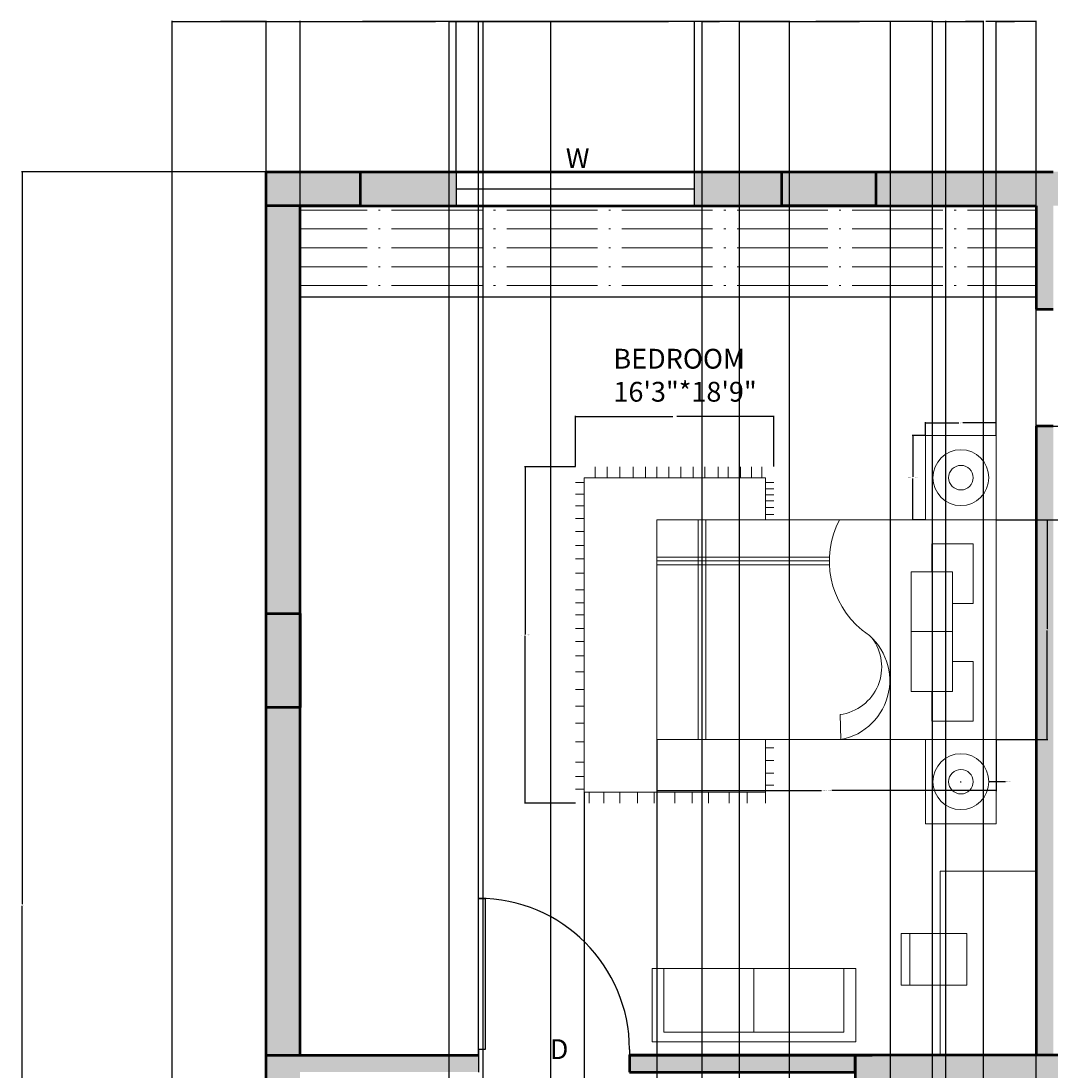
# Model space of a CAD drawing. Units: inches. Extents: x 2494 to 2908, y 1051 to 1885.
# Tile 6 of 7: x 2494 to 2767, y 1607 to 1885. Entities that reach past the tile are written whole.
import ezdxf

# ---------------------------------------------------------------- set-up
doc = ezdxf.new("R2010")
doc.units = ezdxf.units.IN
for name, color, linetype, lineweight in [('A-ANNO-DIMS', 2, 'Continuous', 18), ('A-ANNO-IDEN', 130, 'Continuous', 18), ('A-AREA-IDEN', 130, 'Continuous', 18), ('A-COLS-PATT', 200, 'Continuous', 13), ('A-FLOR-CASE', 230, 'Continuous', 25), ('A-FURN-PATT', 230, 'Continuous', 13), ('A-WALL-PATT', 140, 'Continuous', 13), ('COLUMN', 200, 'Continuous', 50), ('DOOR', 50, 'Continuous', 25), ('FUR', 230, 'Continuous', 18), ('WALL', 140, 'Continuous', 50), ('WIND', 210, 'Continuous', 25)]:
    doc.layers.add(name, color=color, linetype=linetype, lineweight=lineweight)
doc.styles.get("Standard").update_dxf_attribs({"font": 'arial.ttf'})
doc.dimstyles.get("Standard").update_dxf_attribs({"dimtxt": 0.18, "dimasz": 0.18, "dimexe": 0.18, "dimexo": 0.0625, "dimgap": 0.09, "dimtad": 0, "dimtih": 1, "dimtoh": 1, "dimdec": 4, "dimzin": 0, "dimdsep": 46, "dimtxsty": 'Standard', "dimcen": 0.09, "dimadec": 0, "dimazin": 0, "dimtfac": 1, "dimtdec": 4, "dimtofl": 0, "dimtmove": 0, "dimatfit": 3, "dimfxl": 1, "dimtolj": 1, "dimtzin": 0, "dimarcsym": 0})

# ---------------------------------------------------------------- blocks, each defined once
blk = doc.blocks.new('*U2')
for p, q in [((0, 0), (0, -6)), ((40, 0), (40, -6))]:
    blk.add_line(p, q)
blk.add_lwpolyline([(0, 0), (0, 40), (1.75, 40), (1.75, 0)], close=True)
blk.add_arc((0, 0), 40, 0, 90)
blk = doc.blocks.new('BED-DOUBLE')
for p, q in [((10.93, 58.24), (10.93, 0)), ((11.93, 58.24), (11.93, 0)), ((12.93, 58.24), (12.93, 0)), ((45.66, 48.34), (0, 48.34)), ((45.66, 47.34), (0, 47.34)), ((45.66, 46.34), (0, 46.34)), ((67.33, 28.6), (78.31, 28.6)), ((48.68, 0), (48.5, 6.63))]:
    blk.add_line(p, q)
for points in [[(89.88, 0), (0, 0), (0, 58.24), (89.88, 58.24)], [(78.31, 44.44), (67.33, 44.44), (67.33, 12.76), (78.31, 12.76)], [(67.33, 28.6), (78.31, 28.6), (78.31, 44.44), (67.33, 44.44)], [(67.33, 12.76), (78.31, 12.76), (78.31, 28.6), (67.33, 28.6)]]:
    blk.add_lwpolyline(points, close=True)
for points in [[(78.31, 36.06), (83.8, 36.06), (83.8, 51.9), (72.82, 51.9), (72.82, 44.44)], [(72.82, 12.76), (72.82, 4.84), (83.8, 4.84), (83.8, 20.68), (78.31, 20.68)]]:
    blk.add_lwpolyline(points)
for centre, radius, start, end in [((69.31, 47.34), 23.65, 152.5545, 230.8062), ((45.78, 15.63), 15.89, 280.497, 57.3115), ((46.81, 19.24), 12.73, 277.6511, 37.2925)]:
    blk.add_arc(centre, radius, start, end)
blk = doc.blocks.new('NIGHTSTAND-WITH-LAMP')
blk.add_lwpolyline([(18.73, 0), (0, 0), (0, 22.3), (18.73, 22.3)], close=True)
for radius in [7.4, 3.25]:
    blk.add_circle((9.36, 11.15), radius)
blk = doc.blocks.new('RUG-BEDROOM-FRINGED')
for p, q in [((5.18, 86.18), (5.18, 89.12)), ((8.36, 86.18), (8.36, 89.12)), ((11.73, 86.18), (11.73, 89.12)), ((15.23, 86.18), (15.23, 89.12)), ((18.48, 86.18), (18.48, 89.12)), ((21.53, 86.18), (21.53, 89.12)), ((24.71, 86.18), (24.71, 89.12)), ((27.86, 86.18), (27.86, 89.12)), ((31.13, 86.18), (31.13, 89.12)), ((34.27, 86.18), (34.27, 89.12)), ((37.78, 86.18), (37.78, 89.12)), ((40.38, 86.18), (40.38, 89.12)), ((43.7, 86.18), (43.7, 89.12)), ((46.57, 86.18), (46.57, 89.12)), ((49.32, 86.18), (49.32, 89.12)), ((0, 84.95), (2.23, 84.95)), ((50.28, 86.18), (2.23, 86.18)), ((2.23, 86.18), (2.23, 2.94)), ((50.28, 75.11), (50.28, 86.18)), ((50.28, 84.95), (52.51, 84.95)), ((0, 81.88), (2.23, 81.88)), ((50.28, 83.33), (52.51, 83.33)), ((50.28, 81.74), (52.51, 81.74)), ((0, 78.8), (2.23, 78.8)), ((50.28, 80.14), (52.51, 80.14)), ((50.28, 78.33), (52.51, 78.33)), ((0, 75.44), (2.23, 75.44)), ((50.28, 76.54), (52.51, 76.54)), ((0, 71.98), (2.23, 71.98)), ((0, 68.3), (2.23, 68.3)), ((0, 64.75), (2.23, 64.75)), ((0, 60.92), (2.23, 60.92)), ((0, 56.55), (2.23, 56.55)), ((0, 53.1), (2.23, 53.1)), ((0, 49.9), (2.23, 49.9)), ((0, 46.27), (2.23, 46.27)), ((0, 42.87), (2.23, 42.87)), ((0, 39.09), (2.23, 39.09)), ((0, 34.84), (2.23, 34.84)), ((0, 30.1), (2.23, 30.1)), ((0, 25.69), (2.23, 25.69)), ((0, 21.25), (2.23, 21.25)), ((50.28, 2.94), (50.28, 16.87)), ((0, 16.29), (2.23, 16.29)), ((50.28, 14.72), (52.51, 14.72)), ((50.28, 11.34), (52.51, 11.34)), ((0, 10.85), (2.23, 10.85)), ((0, 7.08), (2.23, 7.08)), ((50.28, 7.95), (52.51, 7.95)), ((0, 3.73), (2.23, 3.73)), ((2.23, 2.94), (50.28, 2.94)), ((3.63, 0), (3.63, 2.94)), ((7.47, 0), (7.47, 2.94)), ((11.7, 0), (11.7, 2.94)), ((16.39, 0), (16.39, 2.94)), ((20.78, 0), (20.78, 2.94)), ((26.26, 0), (26.26, 2.94)), ((30.86, 0), (30.86, 2.94)), ((35.17, 0), (35.17, 2.94)), ((40.63, 0), (40.63, 2.94)), ((45.48, 0), (45.48, 2.94)), ((50.28, 4.8), (52.51, 4.8)), ((50.28, 0), (50.28, 2.94))]:
    blk.add_line(p, q)
blk = doc.blocks.new('*D12')
at = {"layer": 'A-ANNO-DIMS', "color": 0, "lineweight": -2, "transparency": 16777216}
for p, q in [((2733.86, 1775.26), (2730.39, 1775.26)), ((2730.57, 1775.08), (2730.57, 1764.29)), ((2730.57, 1753.14), (2730.57, 1763.92)), ((2733.86, 1752.96), (2730.39, 1752.96))]:
    blk.add_line(p, q, dxfattribs=at)
at = {"layer": 'A-ANNO-DIMS', "color": 0, "lineweight": 100, "transparency": 16777216}
for points in [[(2730.54, 1775.08), (2730.6, 1775.08), (2730.57, 1775.26)], [(2730.54, 1753.14), (2730.6, 1753.14), (2730.57, 1752.96)]]:
    blk.add_solid(points, dxfattribs=at)
at = {"layer": 'Defpoints', "color": 0, "lineweight": 100, "transparency": 16777216}
for p in [(2730.57, 1775.26), (2733.92, 1775.26), (2733.92, 1752.96)]:
    blk.add_point(p, dxfattribs=at)
at = {"layer": 'A-ANNO-DIMS', "color": 0, "transparency": 16777216, "insert": (2730.57, 1764.11), "char_height": 0.18, "attachment_point": 5}
blk.add_mtext('\\A1;NIGHTSTAND 22 TYP.', dxfattribs=at)
blk = doc.blocks.new('*D13')
at = {"layer": 'A-ANNO-DIMS', "color": 0, "lineweight": -2, "transparency": 16777216}
for p, q in [((2733.92, 1775.32), (2733.92, 1778.78)), ((2734.1, 1778.6), (2742.76, 1778.6)), ((2752.46, 1778.6), (2743.8, 1778.6)), ((2752.64, 1775.32), (2752.64, 1778.78))]:
    blk.add_line(p, q, dxfattribs=at)
at = {"layer": 'A-ANNO-DIMS', "color": 0, "lineweight": 100, "transparency": 16777216}
for points in [[(2734.1, 1778.63), (2734.1, 1778.57), (2733.92, 1778.6)], [(2752.46, 1778.63), (2752.46, 1778.57), (2752.64, 1778.6)]]:
    blk.add_solid(points, dxfattribs=at)
at = {"layer": 'Defpoints', "color": 0, "lineweight": 100, "transparency": 16777216}
for p in [(2752.64, 1778.6), (2733.92, 1775.26), (2752.64, 1775.26)]:
    blk.add_point(p, dxfattribs=at)
at = {"layer": 'A-ANNO-DIMS', "color": 0, "transparency": 16777216, "insert": (2743.28, 1778.6), "char_height": 0.18, "attachment_point": 5}
blk.add_mtext('\\A1;19 TYP.', dxfattribs=at)
blk = doc.blocks.new('*D14')
at = {"layer": 'A-ANNO-DIMS', "color": 0, "lineweight": -2, "transparency": 16777216}
for p, q in [((2662.76, 1694.66), (2662.76, 1681.06)), ((2752.64, 1694.66), (2752.64, 1681.06)), ((2662.94, 1681.24), (2706.34, 1681.24)), ((2752.46, 1681.24), (2709.07, 1681.24))]:
    blk.add_line(p, q, dxfattribs=at)
at = {"layer": 'A-ANNO-DIMS', "color": 0, "lineweight": 100, "transparency": 16777216}
for points in [[(2662.94, 1681.27), (2662.94, 1681.21), (2662.76, 1681.24)], [(2752.46, 1681.27), (2752.46, 1681.21), (2752.64, 1681.24)]]:
    blk.add_solid(points, dxfattribs=at)
at = {"layer": 'Defpoints', "color": 0, "lineweight": 100, "transparency": 16777216}
for p in [(2662.76, 1694.72), (2752.64, 1694.72), (2752.64, 1681.24)]:
    blk.add_point(p, dxfattribs=at)
at = {"layer": 'A-ANNO-DIMS', "color": 0, "transparency": 16777216, "insert": (2707.7, 1681.24), "char_height": 0.18, "attachment_point": 5}
blk.add_mtext('\\A1;DOUBLE BED 90 TYP.', dxfattribs=at)
blk = doc.blocks.new('*D15')
at = {"layer": 'A-ANNO-DIMS', "color": 0, "lineweight": -2, "transparency": 16777216}
for p, q in [((2752.71, 1752.96), (2766.31, 1752.96)), ((2766.13, 1752.78), (2766.13, 1724.02)), ((2766.13, 1694.9), (2766.13, 1723.66)), ((2752.71, 1694.72), (2766.31, 1694.72))]:
    blk.add_line(p, q, dxfattribs=at)
at = {"layer": 'A-ANNO-DIMS', "color": 0, "lineweight": 100, "transparency": 16777216}
for points in [[(2766.1, 1752.78), (2766.16, 1752.78), (2766.13, 1752.96)], [(2766.1, 1694.9), (2766.16, 1694.9), (2766.13, 1694.72)]]:
    blk.add_solid(points, dxfattribs=at)
at = {"layer": 'Defpoints', "color": 0, "lineweight": 100, "transparency": 16777216}
for p in [(2752.64, 1752.96), (2766.13, 1752.96), (2752.64, 1694.72)]:
    blk.add_point(p, dxfattribs=at)
at = {"layer": 'A-ANNO-DIMS', "color": 0, "transparency": 16777216, "insert": (2766.13, 1723.84), "char_height": 0.18, "attachment_point": 5}
blk.add_mtext('\\A1;58 TYP.', dxfattribs=at)
blk = doc.blocks.new('*D16')
at = {"layer": 'A-ANNO-DIMS', "color": 0, "lineweight": -2, "transparency": 16777216}
for p, q in [((2641.17, 1766.97), (2627.68, 1766.97)), ((2627.86, 1766.79), (2627.86, 1722.59)), ((2627.86, 1678.03), (2627.86, 1722.23)), ((2641.17, 1677.85), (2627.68, 1677.85))]:
    blk.add_line(p, q, dxfattribs=at)
at = {"layer": 'A-ANNO-DIMS', "color": 0, "lineweight": 100, "transparency": 16777216}
for points in [[(2627.83, 1766.79), (2627.89, 1766.79), (2627.86, 1766.97)], [(2627.83, 1678.03), (2627.89, 1678.03), (2627.86, 1677.85)]]:
    blk.add_solid(points, dxfattribs=at)
at = {"layer": 'Defpoints', "color": 0, "lineweight": 100, "transparency": 16777216}
for p in [(2627.86, 1766.97), (2641.23, 1766.97), (2641.23, 1677.85)]:
    blk.add_point(p, dxfattribs=at)
at = {"layer": 'A-ANNO-DIMS', "color": 0, "transparency": 16777216, "insert": (2627.86, 1722.41), "char_height": 0.18, "attachment_point": 5}
blk.add_mtext('\\A1;BEDROOM RUG 89 TYP.', dxfattribs=at)
blk = doc.blocks.new('*D17')
at = {"layer": 'A-ANNO-DIMS', "color": 0, "lineweight": -2, "transparency": 16777216}
for p, q in [((2641.23, 1767.03), (2641.23, 1780.52)), ((2641.41, 1780.34), (2666.96, 1780.34)), ((2693.56, 1780.34), (2668.01, 1780.34)), ((2693.74, 1767.03), (2693.74, 1780.52))]:
    blk.add_line(p, q, dxfattribs=at)
at = {"layer": 'A-ANNO-DIMS', "color": 0, "lineweight": 100, "transparency": 16777216}
for points in [[(2641.41, 1780.37), (2641.41, 1780.31), (2641.23, 1780.34)], [(2693.56, 1780.37), (2693.56, 1780.31), (2693.74, 1780.34)]]:
    blk.add_solid(points, dxfattribs=at)
at = {"layer": 'Defpoints', "color": 0, "lineweight": 100, "transparency": 16777216}
for p in [(2693.74, 1780.34), (2641.23, 1766.97), (2693.74, 1766.97)]:
    blk.add_point(p, dxfattribs=at)
at = {"layer": 'A-ANNO-DIMS', "color": 0, "transparency": 16777216, "insert": (2667.49, 1780.34), "char_height": 0.18, "attachment_point": 5}
blk.add_mtext('\\A1;53 TYP.', dxfattribs=at)
blk = doc.blocks.new('*D22')
at = {"layer": 'A-ANNO-DIMS', "color": 0, "lineweight": -2, "transparency": 16777216}
for p, q in [((2534.4, 1456.72), (2534.4, 1885.09)), ((2534.58, 1884.91), (2546.43, 1884.91)), ((2559.07, 1884.91), (2547.22, 1884.91)), ((2559.25, 1845.22), (2559.25, 1885.09))]:
    blk.add_line(p, q, dxfattribs=at)
at = {"layer": 'A-ANNO-DIMS', "color": 0, "lineweight": 100, "transparency": 16777216}
for points in [[(2534.58, 1884.94), (2534.58, 1884.88), (2534.4, 1884.91)], [(2559.07, 1884.94), (2559.07, 1884.88), (2559.25, 1884.91)]]:
    blk.add_solid(points, dxfattribs=at)
at = {"layer": 'Defpoints', "color": 0, "lineweight": 100, "transparency": 16777216}
for p in [(2559.25, 1884.91), (2559.25, 1845.16), (2534.4, 1456.66)]:
    blk.add_point(p, dxfattribs=at)
at = {"layer": 'A-ANNO-DIMS', "color": 0, "transparency": 16777216, "insert": (2546.83, 1884.91), "char_height": 0.18, "attachment_point": 5}
blk.add_mtext('\\A1;24.85', dxfattribs=at)
blk = doc.blocks.new('*D23')
at = {"layer": 'A-ANNO-DIMS', "color": 0, "lineweight": -2, "transparency": 16777216}
for p, q in [((2559.25, 1845.22), (2559.25, 1885.09)), ((2559.43, 1884.91), (2584.04, 1884.91)), ((2609.43, 1884.91), (2584.82, 1884.91)), ((2609.61, 1845.22), (2609.61, 1885.09))]:
    blk.add_line(p, q, dxfattribs=at)
at = {"layer": 'A-ANNO-DIMS', "color": 0, "lineweight": 100, "transparency": 16777216}
for points in [[(2559.43, 1884.94), (2559.43, 1884.88), (2559.25, 1884.91)], [(2609.43, 1884.94), (2609.43, 1884.88), (2609.61, 1884.91)]]:
    blk.add_solid(points, dxfattribs=at)
at = {"layer": 'Defpoints', "color": 0, "lineweight": 100, "transparency": 16777216}
for p in [(2609.61, 1884.91), (2559.25, 1845.16), (2609.61, 1845.16)]:
    blk.add_point(p, dxfattribs=at)
at = {"layer": 'A-ANNO-DIMS', "color": 0, "transparency": 16777216, "insert": (2584.43, 1884.91), "char_height": 0.18, "attachment_point": 5}
blk.add_mtext('\\A1;50.36', dxfattribs=at)
blk = doc.blocks.new('*D24')
at = {"layer": 'A-ANNO-DIMS', "color": 0, "lineweight": -2, "transparency": 16777216}
for p, q in [((2609.61, 1845.22), (2609.61, 1885.09)), ((2609.79, 1884.91), (2640.79, 1884.91)), ((2672.58, 1884.91), (2641.58, 1884.91)), ((2672.76, 1845.22), (2672.76, 1885.09))]:
    blk.add_line(p, q, dxfattribs=at)
at = {"layer": 'A-ANNO-DIMS', "color": 0, "lineweight": 100, "transparency": 16777216}
for points in [[(2609.79, 1884.94), (2609.79, 1884.88), (2609.61, 1884.91)], [(2672.58, 1884.94), (2672.58, 1884.88), (2672.76, 1884.91)]]:
    blk.add_solid(points, dxfattribs=at)
at = {"layer": 'Defpoints', "color": 0, "lineweight": 100, "transparency": 16777216}
for p in [(2672.76, 1884.91), (2609.61, 1845.16), (2672.76, 1845.16)]:
    blk.add_point(p, dxfattribs=at)
at = {"layer": 'A-ANNO-DIMS', "color": 0, "transparency": 16777216, "insert": (2641.18, 1884.91), "char_height": 0.18, "attachment_point": 5}
blk.add_mtext('\\A1;63.15', dxfattribs=at)
blk = doc.blocks.new('*D27')
at = {"layer": 'A-ANNO-DIMS', "color": 0, "lineweight": -2, "transparency": 16777216}
for p, q in [((2559.19, 1845.16), (2494.47, 1845.16)), ((2494.65, 1844.98), (2494.65, 1651.09)), ((2494.65, 1456.84), (2494.65, 1650.72)), ((2559.19, 1456.66), (2494.47, 1456.66))]:
    blk.add_line(p, q, dxfattribs=at)
at = {"layer": 'A-ANNO-DIMS', "color": 0, "lineweight": 100, "transparency": 16777216}
for points in [[(2494.62, 1844.98), (2494.68, 1844.98), (2494.65, 1845.16)], [(2494.62, 1456.84), (2494.68, 1456.84), (2494.65, 1456.66)]]:
    blk.add_solid(points, dxfattribs=at)
at = {"layer": 'Defpoints', "color": 0, "lineweight": 100, "transparency": 16777216}
for p in [(2494.65, 1845.16), (2559.25, 1845.16), (2559.25, 1456.66)]:
    blk.add_point(p, dxfattribs=at)
at = {"layer": 'A-ANNO-DIMS', "color": 0, "transparency": 16777216, "insert": (2494.65, 1650.91), "char_height": 0.18, "attachment_point": 5}
blk.add_mtext('\\A1;388.5', dxfattribs=at)
blk = doc.blocks.new('*D33')
at = {"layer": 'A-ANNO-DIMS', "color": 0, "lineweight": -2, "transparency": 16777216}
for p, q in [((2697.84, 1155.22), (2697.84, 1885.09)), ((2698.02, 1884.91), (2716.38, 1884.91)), ((2735.54, 1884.91), (2717.17, 1884.91)), ((2735.72, 1155.22), (2735.72, 1885.09))]:
    blk.add_line(p, q, dxfattribs=at)
at = {"layer": 'A-ANNO-DIMS', "color": 0, "lineweight": 100, "transparency": 16777216}
for points in [[(2698.02, 1884.94), (2698.02, 1884.88), (2697.84, 1884.91)], [(2735.54, 1884.94), (2735.54, 1884.88), (2735.72, 1884.91)]]:
    blk.add_solid(points, dxfattribs=at)
at = {"layer": 'Defpoints', "color": 0, "lineweight": 100, "transparency": 16777216}
for p in [(2735.72, 1884.91), (2697.84, 1155.16), (2735.72, 1155.16)]:
    blk.add_point(p, dxfattribs=at)
at = {"layer": 'A-ANNO-DIMS', "color": 0, "transparency": 16777216, "insert": (2716.78, 1884.91), "char_height": 0.18, "attachment_point": 5}
blk.add_mtext('\\A1;37.88', dxfattribs=at)
blk = doc.blocks.new('*D34')
at = {"layer": 'A-ANNO-DIMS', "color": 0, "lineweight": -2, "transparency": 16777216}
for p, q in [((2634.69, 1155.22), (2634.69, 1885.09)), ((2634.87, 1884.91), (2665.87, 1884.91)), ((2697.66, 1884.91), (2666.66, 1884.91)), ((2697.84, 1155.22), (2697.84, 1885.09))]:
    blk.add_line(p, q, dxfattribs=at)
at = {"layer": 'A-ANNO-DIMS', "color": 0, "lineweight": 100, "transparency": 16777216}
for points in [[(2634.87, 1884.94), (2634.87, 1884.88), (2634.69, 1884.91)], [(2697.66, 1884.94), (2697.66, 1884.88), (2697.84, 1884.91)]]:
    blk.add_solid(points, dxfattribs=at)
at = {"layer": 'Defpoints', "color": 0, "lineweight": 100, "transparency": 16777216}
for p in [(2697.84, 1884.91), (2634.69, 1155.16), (2697.84, 1155.16)]:
    blk.add_point(p, dxfattribs=at)
at = {"layer": 'A-ANNO-DIMS', "color": 0, "transparency": 16777216, "insert": (2666.26, 1884.91), "char_height": 0.18, "attachment_point": 5}
blk.add_mtext('\\A1;63.15', dxfattribs=at)
blk = doc.blocks.new('*D35')
at = {"layer": 'A-ANNO-DIMS', "color": 0, "lineweight": -2, "transparency": 16777216}
for p, q in [((2735.72, 1155.22), (2735.72, 1885.09)), ((2735.9, 1884.91), (2749.09, 1884.91)), ((2763.07, 1884.91), (2749.88, 1884.91)), ((2763.25, 1155.22), (2763.25, 1885.09))]:
    blk.add_line(p, q, dxfattribs=at)
at = {"layer": 'A-ANNO-DIMS', "color": 0, "lineweight": 100, "transparency": 16777216}
for points in [[(2735.9, 1884.94), (2735.9, 1884.88), (2735.72, 1884.91)], [(2763.07, 1884.94), (2763.07, 1884.88), (2763.25, 1884.91)]]:
    blk.add_solid(points, dxfattribs=at)
at = {"layer": 'Defpoints', "color": 0, "lineweight": 100, "transparency": 16777216}
for p in [(2763.25, 1884.91), (2735.72, 1155.16), (2763.25, 1155.16)]:
    blk.add_point(p, dxfattribs=at)
at = {"layer": 'A-ANNO-DIMS', "color": 0, "transparency": 16777216, "insert": (2749.49, 1884.91), "char_height": 0.18, "attachment_point": 5}
blk.add_mtext('\\A1;27.53', dxfattribs=at)
blk = doc.blocks.new('*D39')
at = {"layer": 'A-ANNO-DIMS', "color": 0, "lineweight": -2, "transparency": 16777216}
for p, q in [((2568.25, 1611.22), (2568.25, 1885.09)), ((2568.43, 1884.91), (2591.47, 1884.91)), ((2615.31, 1884.91), (2592.27, 1884.91)), ((2615.49, 1611.22), (2615.49, 1885.09))]:
    blk.add_line(p, q, dxfattribs=at)
at = {"layer": 'A-ANNO-DIMS', "color": 0, "lineweight": 100, "transparency": 16777216}
for points in [[(2568.43, 1884.94), (2568.43, 1884.88), (2568.25, 1884.91)], [(2615.31, 1884.94), (2615.31, 1884.88), (2615.49, 1884.91)]]:
    blk.add_solid(points, dxfattribs=at)
at = {"layer": 'Defpoints', "color": 0, "lineweight": 100, "transparency": 16777216}
for p in [(2615.49, 1884.91), (2568.25, 1611.16), (2615.49, 1611.16)]:
    blk.add_point(p, dxfattribs=at)
at = {"layer": 'A-ANNO-DIMS', "color": 0, "transparency": 16777216, "insert": (2591.87, 1884.91), "char_height": 0.18, "attachment_point": 5}
blk.add_mtext('\\A1;47.24', dxfattribs=at)
blk = doc.blocks.new('*D41')
at = {"layer": 'A-ANNO-DIMS', "color": 0, "lineweight": -2, "transparency": 16777216}
for p, q in [((2684.64, 1347.22), (2684.64, 1885.09)), ((2684.82, 1884.91), (2704.42, 1884.91)), ((2724.46, 1884.91), (2704.86, 1884.91)), ((2724.64, 1347.22), (2724.64, 1885.09))]:
    blk.add_line(p, q, dxfattribs=at)
at = {"layer": 'A-ANNO-DIMS', "color": 0, "lineweight": 100, "transparency": 16777216}
for points in [[(2684.82, 1884.94), (2684.82, 1884.88), (2684.64, 1884.91)], [(2724.46, 1884.94), (2724.46, 1884.88), (2724.64, 1884.91)]]:
    blk.add_solid(points, dxfattribs=at)
at = {"layer": 'Defpoints', "color": 0, "lineweight": 100, "transparency": 16777216}
for p in [(2724.64, 1884.91), (2684.64, 1347.16), (2724.64, 1347.16)]:
    blk.add_point(p, dxfattribs=at)
at = {"layer": 'A-ANNO-DIMS', "color": 0, "transparency": 16777216, "insert": (2704.64, 1884.91), "char_height": 0.18, "attachment_point": 5}
blk.add_mtext('\\A1;40', dxfattribs=at)
blk = doc.blocks.new('*D42')
at = {"layer": 'A-ANNO-DIMS', "color": 0, "lineweight": -2, "transparency": 16777216}
for p, q in [((2674.75, 1347.22), (2674.75, 1885.09)), ((2674.93, 1884.91), (2679.3, 1884.91)), ((2684.46, 1884.91), (2680.09, 1884.91)), ((2684.64, 1347.22), (2684.64, 1885.09))]:
    blk.add_line(p, q, dxfattribs=at)
at = {"layer": 'A-ANNO-DIMS', "color": 0, "lineweight": 100, "transparency": 16777216}
for points in [[(2674.93, 1884.94), (2674.93, 1884.88), (2674.75, 1884.91)], [(2684.46, 1884.94), (2684.46, 1884.88), (2684.64, 1884.91)]]:
    blk.add_solid(points, dxfattribs=at)
at = {"layer": 'Defpoints', "color": 0, "lineweight": 100, "transparency": 16777216}
for p in [(2684.64, 1884.91), (2674.75, 1347.16), (2684.64, 1347.16)]:
    blk.add_point(p, dxfattribs=at)
at = {"layer": 'A-ANNO-DIMS', "color": 0, "transparency": 16777216, "insert": (2679.7, 1884.91), "char_height": 0.18, "attachment_point": 5}
blk.add_mtext('\\A1;9.889', dxfattribs=at)
blk = doc.blocks.new('*D48')
at = {"layer": 'A-ANNO-DIMS', "color": 0, "lineweight": -2, "transparency": 16777216}
for p, q in [((2534.4, 1456.72), (2534.4, 1885.09)), ((2534.58, 1884.91), (2604.12, 1884.91)), ((2674.57, 1884.91), (2605.03, 1884.91)), ((2674.75, 1456.72), (2674.75, 1885.09))]:
    blk.add_line(p, q, dxfattribs=at)
at = {"layer": 'A-ANNO-DIMS', "color": 0, "lineweight": 100, "transparency": 16777216}
for points in [[(2534.58, 1884.94), (2534.58, 1884.88), (2534.4, 1884.91)], [(2674.57, 1884.94), (2674.57, 1884.88), (2674.75, 1884.91)]]:
    blk.add_solid(points, dxfattribs=at)
at = {"layer": 'Defpoints', "color": 0, "lineweight": 100, "transparency": 16777216}
for p in [(2674.75, 1884.91), (2534.4, 1456.66), (2674.75, 1456.66)]:
    blk.add_point(p, dxfattribs=at)
at = {"layer": 'A-ANNO-DIMS', "color": 0, "transparency": 16777216, "insert": (2604.58, 1884.91), "char_height": 0.18, "attachment_point": 5}
blk.add_mtext('\\A1;140.35', dxfattribs=at)
blk = doc.blocks.new('*D55')
at = {"layer": 'A-ANNO-DIMS', "color": 0, "lineweight": -2, "transparency": 16777216}
for p, q in [((2739.28, 1530.22), (2739.28, 1885.09)), ((2739.46, 1884.91), (2744.07, 1884.91)), ((2749.1, 1884.91), (2744.49, 1884.91)), ((2749.28, 1530.22), (2749.28, 1885.09))]:
    blk.add_line(p, q, dxfattribs=at)
at = {"layer": 'A-ANNO-DIMS', "color": 0, "lineweight": 100, "transparency": 16777216}
for points in [[(2739.46, 1884.94), (2739.46, 1884.88), (2739.28, 1884.91)], [(2749.1, 1884.94), (2749.1, 1884.88), (2749.28, 1884.91)]]:
    blk.add_solid(points, dxfattribs=at)
at = {"layer": 'Defpoints', "color": 0, "lineweight": 100, "transparency": 16777216}
for p in [(2749.28, 1884.91), (2739.28, 1530.16), (2749.28, 1530.16)]:
    blk.add_point(p, dxfattribs=at)
at = {"layer": 'A-ANNO-DIMS', "color": 0, "transparency": 16777216, "insert": (2744.28, 1884.91), "char_height": 0.18, "attachment_point": 5}
blk.add_mtext('\\A1;10', dxfattribs=at)
blk = doc.blocks.new('*D64')
at = {"layer": 'A-ANNO-DIMS', "color": 0, "lineweight": -2, "transparency": 16777216}
for p, q in [((2607.71, 1563.72), (2607.71, 1885.09)), ((2607.89, 1884.91), (2611.82, 1884.91)), ((2616.54, 1884.91), (2612.61, 1884.91)), ((2616.72, 1552.6), (2616.72, 1885.09))]:
    blk.add_line(p, q, dxfattribs=at)
at = {"layer": 'A-ANNO-DIMS', "color": 0, "lineweight": 100, "transparency": 16777216}
for points in [[(2607.89, 1884.94), (2607.89, 1884.88), (2607.71, 1884.91)], [(2616.54, 1884.94), (2616.54, 1884.88), (2616.72, 1884.91)]]:
    blk.add_solid(points, dxfattribs=at)
at = {"layer": 'Defpoints', "color": 0, "lineweight": 100, "transparency": 16777216}
for p in [(2616.72, 1884.91), (2607.71, 1563.66), (2616.72, 1552.53)]:
    blk.add_point(p, dxfattribs=at)
at = {"layer": 'A-ANNO-DIMS', "color": 0, "transparency": 16777216, "insert": (2612.22, 1884.91), "char_height": 0.18, "attachment_point": 5}
blk.add_mtext('\\A1;9.008', dxfattribs=at)
blk = doc.blocks.new('*D65')
at = {"layer": 'A-ANNO-DIMS', "color": 0, "lineweight": -2, "transparency": 16777216}
for p, q in [((2662.76, 1694.66), (2662.76, 1051.41)), ((2643.46, 1680.73), (2643.46, 1051.41)), ((2643.64, 1051.59), (2652.66, 1051.59)), ((2662.58, 1051.59), (2653.57, 1051.59))]:
    blk.add_line(p, q, dxfattribs=at)
at = {"layer": 'A-ANNO-DIMS', "color": 0, "lineweight": 100, "transparency": 16777216}
for points in [[(2643.64, 1051.62), (2643.64, 1051.56), (2643.46, 1051.59)], [(2662.58, 1051.62), (2662.58, 1051.56), (2662.76, 1051.59)]]:
    blk.add_solid(points, dxfattribs=at)
at = {"layer": 'Defpoints', "color": 0, "lineweight": 100, "transparency": 16777216}
for p in [(2662.76, 1694.72), (2643.46, 1680.79), (2662.76, 1051.59)]:
    blk.add_point(p, dxfattribs=at)
at = {"layer": 'A-ANNO-DIMS', "color": 0, "transparency": 16777216, "insert": (2653.11, 1051.59), "char_height": 0.18, "attachment_point": 5}
blk.add_mtext('\\A1;19.305', dxfattribs=at)
blk = doc.blocks.new('*D66')
at = {"layer": 'A-ANNO-DIMS', "color": 0, "lineweight": -2, "transparency": 16777216}
for p, q in [((2752.64, 1775.32), (2752.64, 1885.09)), ((2752.82, 1884.91), (2757.49, 1884.91)), ((2763.07, 1884.91), (2758.4, 1884.91)), ((2763.25, 1777.79), (2763.25, 1885.09))]:
    blk.add_line(p, q, dxfattribs=at)
at = {"layer": 'A-ANNO-DIMS', "color": 0, "lineweight": 100, "transparency": 16777216}
for points in [[(2752.82, 1884.94), (2752.82, 1884.88), (2752.64, 1884.91)], [(2763.07, 1884.94), (2763.07, 1884.88), (2763.25, 1884.91)]]:
    blk.add_solid(points, dxfattribs=at)
at = {"layer": 'Defpoints', "color": 0, "lineweight": 100, "transparency": 16777216}
for p in [(2763.25, 1884.91), (2763.25, 1777.73), (2752.64, 1775.26)]:
    blk.add_point(p, dxfattribs=at)
at = {"layer": 'A-ANNO-DIMS', "color": 0, "transparency": 16777216, "insert": (2757.95, 1884.91), "char_height": 0.18, "attachment_point": 5}
blk.add_mtext('\\A1;10.607', dxfattribs=at)
blk = doc.blocks.new('*D67')
at = {"layer": 'A-ANNO-DIMS', "color": 0, "lineweight": -2, "transparency": 16777216}
for p, q in [((2767.81, 1777.73), (2908.18, 1777.73)), ((2908, 1777.55), (2908, 1765.52)), ((2908, 1753.14), (2908, 1765.16)), ((2752.71, 1752.96), (2908.18, 1752.96))]:
    blk.add_line(p, q, dxfattribs=at)
at = {"layer": 'A-ANNO-DIMS', "color": 0, "lineweight": 100, "transparency": 16777216}
for points in [[(2907.97, 1777.55), (2908.03, 1777.55), (2908, 1777.73)], [(2907.97, 1753.14), (2908.03, 1753.14), (2908, 1752.96)]]:
    blk.add_solid(points, dxfattribs=at)
at = {"layer": 'Defpoints', "color": 0, "lineweight": 100, "transparency": 16777216}
for p in [(2767.75, 1777.73), (2908, 1777.73), (2752.64, 1752.96)]:
    blk.add_point(p, dxfattribs=at)
at = {"layer": 'A-ANNO-DIMS', "color": 0, "transparency": 16777216, "insert": (2908, 1765.34), "char_height": 0.18, "attachment_point": 5}
blk.add_mtext('\\A1;24.77', dxfattribs=at)
blk = doc.blocks.new('*D68')
at = {"layer": 'A-ANNO-DIMS', "color": 0, "lineweight": -2, "transparency": 16777216}
for p, q in [((2743.19, 1683.57), (2743.37, 1683.57)), ((2743.28, 1683.48), (2743.28, 1683.66)), ((2755.12, 1683.57), (2750.86, 1683.57))]:
    blk.add_line(p, q, dxfattribs=at)
at = {"layer": 'A-ANNO-DIMS', "color": 0, "lineweight": 100, "transparency": 16777216}
blk.add_solid([(2750.86, 1683.6), (2750.86, 1683.54), (2750.68, 1683.57)], dxfattribs=at)
at = {"layer": 'Defpoints', "color": 0, "lineweight": 100, "transparency": 16777216}
for p in [(2735.88, 1683.57), (2750.68, 1683.57)]:
    blk.add_point(p, dxfattribs=at)
at = {"layer": 'A-ANNO-DIMS', "color": 0, "transparency": 16777216, "insert": (2755.88, 1683.57), "char_height": 0.18, "attachment_point": 5}
blk.add_mtext('\\A1;4X ∅14.803', dxfattribs=at)

msp = doc.modelspace()

# ---------------------------------------------------------------- hatches: boundary and pattern name
at = {"layer": 'A-COLS-PATT'}
h = msp.add_hatch(color=256, dxfattribs=at)
h.dxf.hatch_style = 1
h.paths.add_polyline_path([(2584.1612, 1845.1561), (2559.2517, 1845.1561), (2559.2517, 1836.1561), (2584.1612, 1836.1561)])
h.paths.add_polyline_path([(2720.7462, 1845.1561), (2695.8368, 1845.1561), (2695.8368, 1836.1561), (2720.7462, 1836.1561)])
h.paths.add_polyline_path([(2868.2517, 1845.1561), (2843.3423, 1845.1561), (2843.3423, 1836.1561), (2868.2517, 1836.1561)])
h.paths.add_polyline_path([(2568.2517, 1728.1561), (2559.2517, 1728.1561), (2559.2517, 1703.2467), (2568.2517, 1703.2467)])
h.paths.add_polyline_path([(2568.2517, 1564.0885), (2559.2517, 1564.0885), (2559.2517, 1539.1791), (2568.2517, 1539.1791)])
h.paths.add_polyline_path([(2868.2517, 1554.4528), (2859.2517, 1554.4528), (2859.2517, 1529.5434), (2868.2517, 1529.5434)])
h.paths.add_polyline_path([(2806.0841, 1611.1561), (2781.1746, 1611.1561), (2781.1746, 1602.1561), (2806.0841, 1602.1561)])
h.paths.add_polyline_path([(2868.0971, 1611.1561), (2843.1877, 1611.1561), (2843.1877, 1602.1561), (2868.0971, 1602.1561)])
h.paths.add_polyline_path([(2584.1612, 1347.1561), (2559.2517, 1347.1561), (2559.2517, 1338.1561), (2584.1612, 1338.1561)])
h.paths.add_polyline_path([(2868.2517, 1347.1561), (2843.3423, 1347.1561), (2843.3423, 1338.1561), (2868.2517, 1338.1561)])
h.paths.add_polyline_path([(2568.2517, 1180.0656), (2559.2517, 1180.0656), (2559.2517, 1155.1561), (2568.2517, 1155.1561)])
h.paths.add_polyline_path([(2584.1612, 1155.1561), (2559.2517, 1155.1561), (2559.2517, 1146.1561), (2584.1612, 1146.1561)])
h.paths.add_polyline_path([(2868.2517, 1155.1561), (2843.3423, 1155.1561), (2843.3423, 1146.1561), (2868.2517, 1146.1561)])
h.paths.add_polyline_path([(2868.2517, 1180.0656), (2859.2517, 1180.0656), (2859.2517, 1155.1561), (2868.2517, 1155.1561)])
at = {"layer": 'A-FURN-PATT'}
h = msp.add_hatch(dxfattribs=at)
h.set_pattern_fill('ACAD_ISO04W100', color=256)
h.paths.add_polyline_path([(2763.2517, 1836.1561), (2568.2517, 1836.1561), (2568.2517, 1811.916), (2763.2517, 1811.916)])
h.paths.add_polyline_path([(2859.2517, 1836.1561), (2843.3423, 1836.1561), (2832.2996, 1836.1561), (2832.2996, 1687.6561), (2859.2517, 1687.6561)])
h.paths.add_polyline_path([(2859.2517, 1338.1485), (2840.7638, 1338.1485), (2840.7638, 1243.6561), (2859.2517, 1243.6561)])
at = {"layer": 'A-WALL-PATT'}
h = msp.add_hatch(color=256, dxfattribs=at)
h.dxf.hatch_style = 1
h.paths.add_polyline_path([(2609.6092, 1845.1561), (2584.1612, 1845.1561), (2584.1612, 1836.1561), (2609.6092, 1836.1561)])
h.paths.add_polyline_path([(2695.8368, 1845.1561), (2672.7564, 1845.1561), (2672.7564, 1836.1561), (2695.8368, 1836.1561)])
h.paths.add_polyline_path([(2767.7517, 1845.1561), (2720.7462, 1845.1561), (2720.7462, 1836.1561), (2763.2517, 1836.1561), (2763.2517, 1808.7615), (2767.7517, 1808.7615)])
h.paths.add_polyline_path([(2843.3423, 1845.1561), (2767.7517, 1845.1561), (2767.7517, 1836.1561), (2843.3423, 1836.1561)])
h.paths.add_polyline_path([(2568.2517, 1836.1561), (2559.2517, 1836.1561), (2559.2517, 1728.1561), (2568.2517, 1728.1561)])
h.paths.add_polyline_path([(2568.2517, 1703.2467), (2559.2517, 1703.2467), (2559.2517, 1611.1561), (2568.2517, 1611.1561)])
h.paths.add_polyline_path([(2843.1877, 1611.1561), (2819.0012, 1611.1561), (2806.0841, 1611.1561), (2806.0841, 1602.1561), (2843.1877, 1602.1561)])
h.paths.add_polyline_path([(2805.2517, 1602.1561), (2796.2517, 1602.1561), (2796.2517, 1591.2367), (2805.2517, 1591.2367)])
h = msp.add_hatch(color=256, dxfattribs=at)
h.dxf.hatch_style = 1
h.paths.add_polyline_path([(2868.2517, 1836.1561), (2859.2517, 1836.1561), (2859.2517, 1611.1561), (2868.2517, 1611.1561)])
h.paths.add_polyline_path([(2715.2517, 1611.1561), (2655.4916, 1611.1561), (2655.4916, 1606.6561), (2715.2517, 1606.6561)])
h.paths.add_polyline_path([(2781.1746, 1611.1561), (2776.9029, 1611.1561), (2715.2517, 1611.1561), (2715.2517, 1606.6561), (2715.2517, 1602.1561), (2781.1746, 1602.1561)])
h.paths.add_polyline_path([(2868.0971, 1602.1561), (2859.2517, 1602.1561), (2859.2517, 1554.4528), (2868.0971, 1554.4528)])
h.paths.add_polyline_path([(2868.2517, 1529.5434), (2859.2517, 1529.5434), (2859.2517, 1347.1561), (2868.2517, 1347.1561)])
h.paths.add_polyline_path([(2868.2517, 1338.1561), (2859.2517, 1338.1561), (2859.2517, 1243.6561), (2868.2517, 1243.6561)])
h.paths.add_polyline_path([(2568.2517, 1338.1561), (2559.2517, 1338.1561), (2559.2517, 1180.0656), (2568.2517, 1180.0656)])
h.paths.add_polyline_path([(2735.7191, 1155.1561), (2697.838, 1155.1561), (2697.838, 1146.1561), (2735.7191, 1146.1561), (2735.7191, 1151.0155)])
h = msp.add_hatch(color=256, dxfattribs=at)
h.dxf.hatch_style = 1
h.paths.add_polyline_path([(2767.7517, 1777.7287), (2763.2517, 1777.7287), (2763.2517, 1611.1561), (2767.7517, 1611.1561), (2767.7517, 1683.1561)])
h = msp.add_hatch(color=256, dxfattribs=at)
h.dxf.hatch_style = 1
h.paths.add_polyline_path([(2805.2517, 1547.9123), (2796.2517, 1547.9123), (2796.2517, 1530.1561), (2859.2517, 1530.1561), (2859.2517, 1539.1561), (2805.2517, 1539.1561)])
h.paths.add_polyline_path([(2568.2517, 1606.6561), (2615.4916, 1606.6561), (2615.4916, 1611.1561), (2559.2517, 1611.1561), (2559.2517, 1564.0885), (2568.2517, 1564.0885)])
h.paths.add_polyline_path([(2568.2517, 1539.1791), (2559.2517, 1539.1791), (2559.2517, 1456.6561), (2534.4016, 1456.6561), (2534.4016, 1338.1561), (2559.2517, 1338.1561), (2559.2517, 1342.6561), (2543.4016, 1342.6561), (2543.4016, 1452.1561), (2559.2517, 1452.1561), (2568.2517, 1452.1561), (2674.7517, 1452.1561), (2674.7517, 1456.6561), (2568.2517, 1456.6561)])
h.paths.add_polyline_path([(2684.6403, 1347.1561), (2674.7517, 1347.1561), (2584.1612, 1347.1561), (2584.1612, 1338.1561), (2684.6403, 1338.1561), (2684.6403, 1341.1561)])
h.paths.add_polyline_path([(2843.3423, 1347.1561), (2832.3482, 1347.1561), (2832.3482, 1338.1485), (2843.3423, 1338.1485)])
h.paths.add_polyline_path([(2634.6908, 1155.1561), (2584.1612, 1155.1561), (2584.1612, 1146.1561), (2634.6908, 1146.1561)])
h.paths.add_polyline_path([(2783.7833, 1155.1561), (2772.2517, 1155.1561), (2772.2517, 1146.1561), (2783.7833, 1146.1561)])
h.paths.add_polyline_path([(2843.3423, 1155.1561), (2819.0012, 1155.1561), (2811.9091, 1155.1561), (2811.9091, 1146.1561), (2843.3423, 1146.1561)])
h.paths.add_polyline_path([(2868.2517, 1243.6561), (2859.2517, 1243.6561), (2859.2517, 1239.1561), (2859.2517, 1180.0656), (2868.2517, 1180.0656)])

# ---------------------------------------------------------------- linework, layer by layer
at = {"layer": 'A-FLOR-CASE'}
msp.add_line((2763.2517, 1811.916), (2568.2517, 1811.916), dxfattribs=at)
at = {"layer": 'COLUMN'}
for points in [[(2559.2517, 1845.1561), (2584.1612, 1845.1561), (2584.1612, 1836.1561), (2559.2517, 1836.1561)], [(2695.8368, 1845.1561), (2720.7462, 1845.1561), (2720.7462, 1836.1561), (2695.8368, 1836.1561)], [(2568.2517, 1728.1561), (2568.2517, 1703.2467), (2559.2517, 1703.2467), (2559.2517, 1728.1561)]]:
    msp.add_lwpolyline(points, close=True, dxfattribs=at)
at = {"layer": 'FUR'}
for p, q in [((2729.7209, 1629.6955), (2729.7209, 1643.3262)), ((2664.6153, 1634.1023), (2664.6153, 1617.2492)), ((2688.461, 1634.1023), (2688.4465, 1617.2492)), ((2712.2777, 1617.2492), (2712.2777, 1634.1023)), ((2664.6153, 1617.2492), (2712.2777, 1617.2492))]:
    msp.add_line(p, q, dxfattribs=at)
for points in [[(2763.2517, 1611.1561), (2737.7892, 1611.1561), (2737.7892, 1659.8599), (2763.2517, 1659.8599)], [(2744.8627, 1643.3262), (2727.4721, 1643.3262), (2727.4721, 1629.6955), (2744.8627, 1629.6955)], [(2661.5043, 1614.638), (2715.4177, 1614.638), (2715.4177, 1634.1023), (2661.5043, 1634.1023)]]:
    msp.add_lwpolyline(points, close=True, dxfattribs=at)
at = {"layer": 'WALL'}
for p, q in [((2559.2517, 1611.1561), (2559.2517, 1845.1561)), ((2559.2517, 1845.1561), (2767.7517, 1845.1561)), ((2568.2517, 1611.1561), (2568.2517, 1836.1561)), ((2568.2517, 1836.1561), (2763.2517, 1836.1561)), ((2763.2517, 1836.1561), (2763.2517, 1808.7615)), ((2763.2517, 1777.7287), (2763.2517, 1611.1561)), ((2559.2517, 1456.6561), (2559.2517, 1611.1561)), ((2559.2517, 1611.1561), (2615.4916, 1611.1561)), ((2655.4916, 1611.1561), (2719.7517, 1611.1561)), ((2868.2517, 1611.1561), (2719.7517, 1611.1561))]:
    msp.add_line(p, q, dxfattribs=at)
for points in [[(2763.2517, 1808.7615), (2767.7517, 1808.7615)], [(2767.7517, 1777.7287), (2763.2517, 1777.7287)]]:
    msp.add_lwpolyline(points, dxfattribs=at)
for points in [[(2655.4916, 1606.6561), (2715.2517, 1606.6561), (2715.2517, 1611.1561), (2655.4916, 1611.1561)], [(2715.2517, 1602.1561), (2781.1746, 1602.1561), (2781.1746, 1611.1561), (2715.2517, 1611.1561)]]:
    msp.add_lwpolyline(points, close=True, dxfattribs=at)
at = {"layer": 'WIND'}
msp.add_line((2609.6092, 1840.6561), (2672.7564, 1840.6561), dxfattribs=at)
msp.add_lwpolyline([(2609.6092, 1836.1561), (2672.7564, 1836.1561), (2672.7564, 1845.1561), (2609.6092, 1845.1561)], close=True, dxfattribs=at)

# ---------------------------------------------------------------- block references
at = {"layer": 'DOOR'}
msp.add_blockref('*U2', (2615.4916, 1612.6561), dxfattribs=at)
at = {"layer": 'FUR'}
for name, p in [('NIGHTSTAND-WITH-LAMP', (2733.918, 1752.9567)), ('RUG-BEDROOM-FRINGED', (2641.229, 1677.8487)), ('BED-DOUBLE', (2662.765, 1694.7187)), ('NIGHTSTAND-WITH-LAMP', (2733.918, 1672.4178))]:
    msp.add_blockref(name, p, dxfattribs=at)

# ---------------------------------------------------------------- texts
at = {"layer": 'A-ANNO-IDEN', "char_height": 5.2482, "attachment_point": 1}
for s, insert in [('W', (2638.6253, 1851.3687)), ('D', (2634.3953, 1615.3356))]:
    msp.add_mtext_dynamic_manual_height_columns(s, width=250.978097, gutter_width=26.2409, heights=[0], dxfattribs=dict(at, insert=insert))
at = {"layer": 'A-AREA-IDEN', "insert": (2651.2477, 1798.2412), "char_height": 5.248177, "attachment_point": 1}
msp.add_mtext_dynamic_manual_height_columns('BEDROOM\\P16\'3"*18\'9"', width=250.978097, gutter_width=26.2409, heights=[0], dxfattribs=at)

# ---------------------------------------------------------------- dimensions: what is measured, and where the dimension line sits
at = {"layer": 'A-ANNO-DIMS'}
for base, p1, p2, override, picture, middle in [((2559.2517, 1884.9061), (2534.4016, 1456.6561), (2559.2517, 1845.1561), {"dimdec": 2, "dimlfac": 1, "dimrnd": 0, "dimzin": 0, "dimdsep": 46, "dimlunit": 2}, '*D22', (2546.8267, 1884.9061)), ((2674.7517, 1884.9061), (2534.4016, 1456.6561), (2674.7517, 1456.6561), {"dimdec": 2, "dimlfac": 1, "dimrnd": 0, "dimzin": 0, "dimdsep": 46, "dimlunit": 2}, '*D48', (2604.5767, 1884.9061)), ((2609.6092, 1884.9061), (2559.2517, 1845.1561), (2609.6092, 1845.1561), {"dimdec": 2, "dimlfac": 1, "dimrnd": 0, "dimzin": 0, "dimdsep": 46, "dimlunit": 2}, '*D23', (2584.4305, 1884.9061)), ((2615.4916, 1884.9061), (2568.2517, 1611.1561), (2615.4916, 1611.1561), {"dimdec": 2, "dimlfac": 1, "dimrnd": 0, "dimzin": 0, "dimdsep": 46, "dimlunit": 2}, '*D39', (2591.8716, 1884.9061)), ((2616.7213, 1884.9061), (2607.7136, 1563.6591), (2616.7213, 1552.5335), {"dimdec": 3, "dimlfac": 1, "dimrnd": 0, "dimzin": 0, "dimdsep": 46, "dimlunit": 2}, '*D64', (2612.2175, 1884.9061)), ((2672.7564, 1884.9061), (2609.6092, 1845.1561), (2672.7564, 1845.1561), {"dimdec": 2, "dimlfac": 1, "dimrnd": 0, "dimzin": 0, "dimdsep": 46, "dimlunit": 2}, '*D24', (2641.1828, 1884.9061)), ((2697.838, 1884.9061), (2634.6908, 1155.1561), (2697.838, 1155.1561), {"dimdec": 2, "dimlfac": 1, "dimrnd": 0, "dimzin": 0, "dimdsep": 46, "dimlunit": 2}, '*D34', (2666.2644, 1884.9061)), ((2684.6403, 1884.9061), (2674.7517, 1347.1561), (2684.6403, 1347.1561), {"dimdec": 3, "dimlfac": 1, "dimrnd": 0, "dimzin": 0, "dimdsep": 46, "dimlunit": 2}, '*D42', (2679.696, 1884.9061)), ((2724.6403, 1884.9061), (2684.6403, 1347.1561), (2724.6403, 1347.1561), {"dimdec": 0, "dimlfac": 1, "dimrnd": 0, "dimzin": 0, "dimdsep": 46, "dimlunit": 2}, '*D41', (2704.6403, 1884.9061)), ((2735.7191, 1884.9061), (2697.838, 1155.1561), (2735.7191, 1155.1561), {"dimdec": 2, "dimlfac": 1, "dimrnd": 0, "dimzin": 0, "dimdsep": 46, "dimlunit": 2}, '*D33', (2716.7785, 1884.9061)), ((2763.2517, 1884.9061), (2735.7191, 1155.1561), (2763.2517, 1155.1561), {"dimdec": 2, "dimlfac": 1, "dimrnd": 0, "dimzin": 0, "dimdsep": 46, "dimlunit": 2}, '*D35', (2749.4854, 1884.9061)), ((2749.2763, 1884.9061), (2739.2763, 1530.1561), (2749.2763, 1530.1561), {"dimdec": 0, "dimlfac": 1, "dimrnd": 0, "dimzin": 0, "dimdsep": 46, "dimlunit": 2}, '*D55', (2744.2763, 1884.9061)), ((2763.2517, 1884.9061), (2752.6447, 1775.2579), (2763.2517, 1777.7287), {"dimdec": 3, "dimlfac": 1, "dimrnd": 0, "dimzin": 0, "dimdsep": 46, "dimlunit": 2}, '*D66', (2757.9482, 1884.9061)), ((2662.7647, 1051.5937), (2643.4597, 1680.7919), (2662.7647, 1694.719), {"dimdec": 3, "dimlfac": 1, "dimrnd": 0, "dimzin": 0, "dimdsep": 46, "dimlunit": 2}, '*D65', (2653.1122, 1051.5937))]:
    dim = msp.add_linear_dim(base=base, p1=p1, p2=p2, dimstyle='Standard', override=override, dxfattribs=at)
    dim.commit()
    dim.dimension.update_dxf_attribs({"geometry": picture, "text_midpoint": middle})
for base, p1, p2, override, picture, middle in [((2494.6516, 1845.1561), (2559.2517, 1456.6561), (2559.2517, 1845.1561), {"dimdec": 1, "dimlfac": 1, "dimrnd": 0, "dimzin": 0, "dimdsep": 46, "dimlunit": 2}, '*D27', (2494.6516, 1650.9061)), ((2908.0017, 1777.7287), (2752.6447, 1752.9565), (2767.7517, 1777.7287), {"dimdec": 2, "dimlfac": 1, "dimrnd": 0, "dimzin": 0, "dimdsep": 46, "dimlunit": 2}, '*D67', (2908.0017, 1765.3426))]:
    dim = msp.add_linear_dim(base=base, p1=p1, p2=p2, angle=90, dimstyle='Standard', override=override, dxfattribs=at)
    dim.commit()
    dim.dimension.update_dxf_attribs({"geometry": picture, "text_midpoint": middle})
for base, p1, p2, text, picture, middle in [((2693.7416, 1780.3384), (2641.2294, 1766.9702), (2693.7416, 1766.9702), '<> TYP.', '*D17', (2667.4855, 1780.3384)), ((2752.6447, 1778.6031), (2733.918, 1775.2579), (2752.6447, 1775.2579), '<> TYP.', '*D13', (2743.2813, 1778.6031)), ((2752.6447, 1681.237), (2662.7647, 1694.719), (2752.6447, 1694.719), 'DOUBLE BED <> TYP.', '*D14', (2707.7047, 1681.237))]:
    dim = msp.add_linear_dim(base=base, p1=p1, p2=p2, text=text, dimstyle='Standard', override={"dimdec": 0, "dimlfac": 1, "dimrnd": 0, "dimzin": 0, "dimdsep": 46, "dimlunit": 2}, dxfattribs=at)
    dim.commit()
    dim.dimension.update_dxf_attribs({"geometry": picture, "text_midpoint": middle})
for base, p1, p2, text, picture, middle in [((2730.5728, 1775.2579), (2733.918, 1752.9565), (2733.918, 1775.2579), 'NIGHTSTAND <> TYP.', '*D12', (2730.5728, 1764.1072)), ((2627.8612, 1766.9702), (2641.2294, 1677.849), (2641.2294, 1766.9702), 'BEDROOM RUG <> TYP.', '*D16', (2627.8612, 1722.4096)), ((2766.1267, 1752.9565), (2752.6447, 1694.719), (2752.6447, 1752.9565), '<> TYP.', '*D15', (2766.1267, 1723.8377))]:
    dim = msp.add_linear_dim(base=base, p1=p1, p2=p2, angle=90, text=text, dimstyle='Standard', override={"dimdec": 0, "dimlfac": 1, "dimrnd": 0, "dimzin": 0, "dimdsep": 46, "dimlunit": 2}, dxfattribs=at)
    dim.commit()
    dim.dimension.update_dxf_attribs({"geometry": picture, "text_midpoint": middle})
dim = msp.add_diameter_dim_2p(p1=(2735.8798, 1683.5666), p2=(2750.6829, 1683.57), text='4X <>', dimstyle='Standard', override={"dimdec": 3, "dimlfac": 1, "dimrnd": 0, "dimzin": 0, "dimdsep": 46, "dimlunit": 2}, dxfattribs=at)
dim.commit()
dim.dimension.update_dxf_attribs({"geometry": '*D68', "text_midpoint": (2755.1238, 1683.571), "dimtype": 163})

doc.saveas('drawing.dxf')
